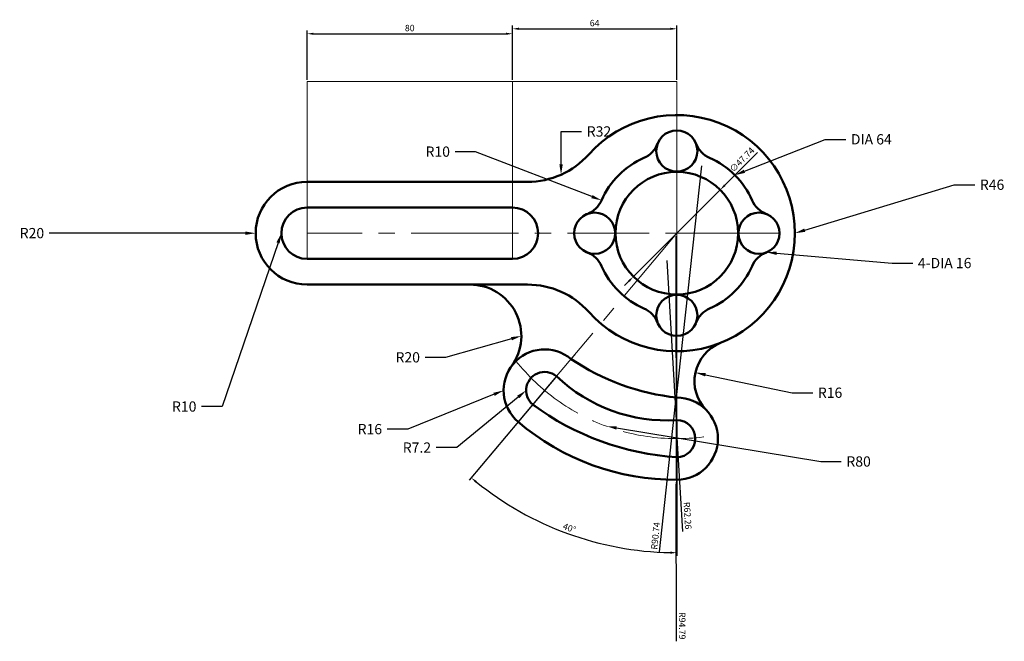
# Model space of a CAD drawing. Units: millimetres. Extents: x 2836 to 3220, y 1446 to 1688.
import ezdxf
from ezdxf import colors
from ezdxf.entities.mleader import LeaderData, LeaderLine
from ezdxf.math import Vec2, Vec3

# ---------------------------------------------------------------- set-up
doc = ezdxf.new("R2010")
doc.units = ezdxf.units.MM
doc.linetypes.add('CENTER', pattern=[50.8, 31.75, -6.35, 6.35, -6.35])
for name, color, linetype, lineweight in [('M-CNTR', 4, 'CENTER', 18), ('M-CONS', 8, 'Continuous', 13), ('M-DIMS', 2, 'Continuous', 25), ('M-OUTL', 7, 'Continuous', 50)]:
    doc.layers.add(name, color=color, linetype=linetype, lineweight=lineweight)
doc.styles.get("Standard").update_dxf_attribs({"font": 'arial.ttf'})
doc.dimstyles.new('ISO-25', dxfattribs={"dimtxt": 2.5, "dimasz": 2.5, "dimexe": 1.25, "dimexo": 0.625, "dimtad": 1, "dimtxsty": 'Standard', "dimcen": 2.5, "dimadec": 0, "dimazin": 0, "dimtfac": 1, "dimtmove": 0, "dimatfit": 3, "dimfxl": 1, "dimarcsym": 0})

# ---------------------------------------------------------------- blocks, each defined once
blk = doc.blocks.new('*U1')
blk.add_circle((0, 0), 8)
blk = doc.blocks.new('*U2')
at = {"layer": 'M-OUTL', "color": 0, "linetype": 'ByBlock', "lineweight": -2, "transparency": 16777216}
blk.add_blockref('*U1', (3092.05, 1637.01), dxfattribs=at)
for p, rotation in [((3060.05, 1605.01), 90), ((3124.05, 1605.01), 270), ((3092.05, 1573.01), 180)]:
    blk.add_blockref('*U1', p, dxfattribs=dict(at, rotation=rotation))
blk = doc.blocks.new('*D3')
at = {"layer": 'Defpoints', "color": 0, "transparency": 16777216}
for p in [(3028.05, 1682.68), (2948.05, 1664.13), (3028.05, 1664.13)]:
    blk.add_point(p, dxfattribs=at)
at = {"layer": 'M-DIMS', "color": 0, "lineweight": -2, "transparency": 16777216}
for p, q in [((2948.05, 1664.76), (2948.05, 1683.93)), ((3028.05, 1664.76), (3028.05, 1683.93)), ((2950.55, 1682.68), (3025.55, 1682.68))]:
    blk.add_line(p, q, dxfattribs=at)
at = {"layer": 'M-DIMS', "color": 0, "transparency": 16777216}
for points in [[(2950.55, 1683.09), (2950.55, 1682.26), (2948.05, 1682.68)], [(3025.55, 1683.09), (3025.55, 1682.26), (3028.05, 1682.68)]]:
    blk.add_solid(points, dxfattribs=at)
at = {"layer": 'M-DIMS', "color": 0, "transparency": 16777216, "insert": (2988.05, 1684.58), "char_height": 2.5, "attachment_point": 5}
blk.add_mtext('80', dxfattribs=at)
blk = doc.blocks.new('*D4')
at = {"layer": 'Defpoints', "color": 0, "transparency": 16777216}
for p in [(3092.05, 1684.61), (3028.05, 1664.13), (3092.05, 1664.13)]:
    blk.add_point(p, dxfattribs=at)
at = {"layer": 'M-DIMS', "color": 0, "lineweight": -2, "transparency": 16777216}
for p, q in [((3028.05, 1664.76), (3028.05, 1685.86)), ((3030.55, 1684.61), (3089.55, 1684.61)), ((3092.05, 1664.76), (3092.05, 1685.86))]:
    blk.add_line(p, q, dxfattribs=at)
at = {"layer": 'M-DIMS', "color": 0, "transparency": 16777216}
for points in [[(3030.55, 1685.03), (3030.55, 1684.19), (3028.05, 1684.61)], [(3089.55, 1685.03), (3089.55, 1684.19), (3092.05, 1684.61)]]:
    blk.add_solid(points, dxfattribs=at)
at = {"layer": 'M-DIMS', "color": 0, "transparency": 16777216, "insert": (3060.05, 1686.51), "char_height": 2.5, "attachment_point": 5}
blk.add_mtext('64', dxfattribs=at)
blk = doc.blocks.new('*D5')
at = {"layer": 'Defpoints', "color": 0, "transparency": 16777216}
for p in [(3092.05, 1605.01), (3092.05, 1559.01), (3045.21, 1549.28), (3092.05, 1532.21), (3036.15, 1493.86)]:
    blk.add_point(p, dxfattribs=at)
at = {"layer": 'M-DIMS', "color": 0, "lineweight": -2, "transparency": 16777216}
for p, q in [((3044.81, 1548.8), (3011.19, 1508.81)), ((3092.05, 1531.59), (3092.05, 1479.34))]:
    blk.add_line(p, q, dxfattribs=at)
blk.add_arc((3092.05, 1605.01), 124.42, 231.1062, 268.8487, dxfattribs=at)
at = {"layer": 'M-DIMS', "color": 0, "transparency": 16777216}
for points in [[(3013.66, 1507.85), (3014.19, 1508.5), (3012, 1509.76)], [(3089.55, 1481.04), (3089.54, 1480.2), (3092.05, 1480.59)]]:
    blk.add_solid(points, dxfattribs=at)
at = {"layer": 'M-DIMS', "color": 0, "transparency": 16777216, "insert": (3050.1, 1489.9), "char_height": 2.5, "attachment_point": 5, "rotation": 339.9775}
blk.add_mtext('40°', dxfattribs=at)
blk = doc.blocks.new('FLANGE-SCALLOP-R32')
for centre, radius, start, end in [((-3.61, 18.1), 10, 23.5565, 68.8316), ((34.89, 34.89), 32, 203.5565, 246.4435), ((18.1, -3.61), 10, 21.1684, 66.4435)]:
    blk.add_arc(centre, radius, start, end)
blk = doc.blocks.new('*D7')
at = {"layer": 'Defpoints', "color": 0, "transparency": 16777216}
for p in [(3108.93, 1621.89), (3075.17, 1588.14)]:
    blk.add_point(p, dxfattribs=at)
at = {"layer": 'M-DIMS', "color": 0, "lineweight": -2, "transparency": 16777216}
for p, q in [((3123.44, 1636.4), (3110.7, 1623.66)), ((3075.17, 1588.14), (3108.93, 1621.89)), ((3073.4, 1586.37), (3071.63, 1584.6))]:
    blk.add_line(p, q, dxfattribs=at)
at = {"layer": 'M-DIMS', "color": 0, "transparency": 16777216}
for points in [[(3110.4, 1623.95), (3110.99, 1623.36), (3108.93, 1621.89)], [(3073.11, 1586.66), (3073.7, 1586.07), (3075.17, 1588.14)]]:
    blk.add_solid(points, dxfattribs=at)
at = {"layer": 'M-DIMS', "color": 0, "transparency": 16777216, "insert": (3117.66, 1633.41), "char_height": 2.5, "attachment_point": 5, "rotation": 44.9932}
blk.add_mtext('∅47.74', dxfattribs=at)
blk = doc.blocks.new('*D8')
at = {"layer": 'Defpoints', "color": 0, "transparency": 16777216}
for p in [(3091.61, 1603.8), (3091.82, 1509.01)]:
    blk.add_point(p, dxfattribs=at)
at = {"layer": 'M-DIMS', "color": 0, "lineweight": -2, "transparency": 16777216}
for p, q in [((3091.61, 1603.8), (3091.82, 1509.01)), ((3091.96, 1446.1), (3091.83, 1506.51))]:
    blk.add_line(p, q, dxfattribs=at)
at = {"layer": 'M-DIMS', "color": 0, "transparency": 16777216}
blk.add_solid([(3092.24, 1506.51), (3091.41, 1506.51), (3091.82, 1509.01)], dxfattribs=at)
at = {"layer": 'M-DIMS', "color": 0, "transparency": 16777216, "insert": (3093.85, 1452.14), "char_height": 2.5, "attachment_point": 5, "rotation": 270.1296}
blk.add_mtext('R94.79', dxfattribs=at)
blk = doc.blocks.new('*D9')
at = {"layer": 'Defpoints', "color": 0, "transparency": 16777216}
for p in [(3101.61, 1631.25), (3091.82, 1541.04)]:
    blk.add_point(p, dxfattribs=at)
at = {"layer": 'M-DIMS', "color": 0, "lineweight": -2, "transparency": 16777216}
for p, q in [((3101.61, 1631.25), (3091.82, 1541.04)), ((3085.3, 1480.91), (3091.55, 1538.55))]:
    blk.add_line(p, q, dxfattribs=at)
at = {"layer": 'M-DIMS', "color": 0, "transparency": 16777216}
blk.add_solid([(3091.14, 1538.6), (3091.97, 1538.51), (3091.82, 1541.04)], dxfattribs=at)
at = {"layer": 'M-DIMS', "color": 0, "transparency": 16777216, "insert": (3084.06, 1487.12), "char_height": 2.5, "attachment_point": 5, "rotation": 83.8079}
blk.add_mtext('R90.74', dxfattribs=at)
blk = doc.blocks.new('*D10')
at = {"layer": 'Defpoints', "color": 0, "transparency": 16777216}
for p in [(3088.16, 1594.35), (3091.82, 1532.2)]:
    blk.add_point(p, dxfattribs=at)
at = {"layer": 'M-DIMS', "color": 0, "lineweight": -2, "transparency": 16777216}
for p, q in [((3088.16, 1594.35), (3091.82, 1532.2)), ((3094.37, 1488.88), (3091.97, 1529.7))]:
    blk.add_line(p, q, dxfattribs=at)
at = {"layer": 'M-DIMS', "color": 0, "transparency": 16777216}
blk.add_solid([(3092.38, 1529.73), (3091.55, 1529.68), (3091.82, 1532.2)], dxfattribs=at)
at = {"layer": 'M-DIMS', "color": 0, "transparency": 16777216, "insert": (3095.91, 1495.02), "char_height": 2.5, "attachment_point": 5, "rotation": 273.3663}
blk.add_mtext('R62.26', dxfattribs=at)

msp = doc.modelspace()

# ---------------------------------------------------------------- linework, layer by layer
at = {"layer": 'M-CNTR'}
for p, q in [((3092.049, 1605.013), (3092.049, 1664.134)), ((3092.049, 1664.134), (3092.049, 1549.257)), ((3092.049, 1549.257), (3092.049, 1606.695)), ((3020.316, 1605.013), (2948.049, 1605.013)), ((3132.049, 1605.013), (3020.316, 1605.013)), ((3092.049, 1605.013), (3045.21, 1549.281)), ((3092.049, 1605.013), (3132.049, 1605.013)), ((3052.59, 1558.063), (3050.872, 1556.018)), ((3092.049, 1559.013), (3092.049, 1532.213)), ((3045.21, 1549.281), (3030.283, 1531.521)), ((3092.049, 1532.213), (3092.049, 1509.013))]:
    msp.add_line(p, q, dxfattribs=at)
msp.add_arc((3092.049, 1605.013), 80, 218.47659, 281.47834, dxfattribs=at)
at = {"layer": 'M-CONS'}
for p, q in [((3028.049, 1664.134), (2948.049, 1664.134)), ((2948.049, 1664.134), (2948.049, 1595.013)), ((3092.049, 1664.134), (3028.049, 1664.134)), ((3028.049, 1664.134), (3028.049, 1595.013))]:
    msp.add_line(p, q, dxfattribs=at)
msp.add_arc((3092.049, 1605.013), 80, 194.47751, 194.66108, dxfattribs=at)
at = {"layer": 'M-OUTL'}
for p, q in [((2948.049, 1625.013), (3033.911, 1625.013)), ((2948.049, 1615.013), (3028.049, 1615.013)), ((2948.049, 1595.013), (3028.049, 1595.013)), ((2948.049, 1585.013), (3033.911, 1585.013))]:
    msp.add_line(p, q, dxfattribs=at)
msp.add_circle((3092.049, 1605.013), 23.868, dxfattribs=at)
for centre, radius, start, end in [((3092.049, 1605.013), 46, 221.81031, 138.18969), ((3033.911, 1657.013), 32, 270, 318.18969), ((2948.049, 1605.013), 20, 90, 270), ((2948.049, 1605.013), 10, 90, 270), ((3028.049, 1605.013), 10, 270, 90), ((3011.513, 1565.013), 20, 323.83691, 90), ((3033.911, 1553.013), 32, 41.81031, 90), ((3114.926, 1547.388), 16, 111.65301, 224.36436), ((3040.577, 1543.769), 16, 49.95493, 229.95493), ((3101.609, 1631.247), 90.739, 236.00275, 263.95218), ((3040.577, 1543.769), 7.2, 49.95493, 237.73801), ((3088.164, 1594.354), 62.262, 226.37816, 273.57677), ((3098.739, 1623.373), 105.773, 233.58177, 266.37316), ((3092.049, 1525.013), 16, 270, 90), ((3091.606, 1603.797), 94.786, 229.68718, 270.26775), ((3092.049, 1525.013), 7.2, 270, 90)]:
    msp.add_arc(centre, radius, start, end, dxfattribs=at)

# ---------------------------------------------------------------- block references
for name, p in [('*U2', (0, 0)), ('FLANGE-SCALLOP-R32', (3057.16, 1570.124))]:
    msp.add_blockref(name, p, dxfattribs=at)
for p, rotation in [((3057.16, 1639.901), 270.0000000000019), ((3126.937, 1639.901), 180), ((3126.937, 1570.124), 90.00000000000095)]:
    msp.add_blockref('FLANGE-SCALLOP-R32', p, dxfattribs=dict(at, rotation=rotation))

# ---------------------------------------------------------------- dimensions: what is measured, and where the dimension line sits
at = {"layer": 'M-DIMS'}
for base, p1, p2, picture, middle in [((3092.049, 1684.609), (3028.049, 1664.134), (3092.049, 1664.134), '*D4', (3060.049, 1686.51)), ((3028.049, 1682.677), (2948.049, 1664.134), (3028.049, 1664.134), '*D3', (2988.049, 1684.578))]:
    dim = msp.add_linear_dim(base=base, p1=p1, p2=p2, dimstyle='ISO-25', override={"dimclrd": 0, "dimclre": 0, "dimclrt": 0}, dxfattribs=at)
    dim.commit()
    dim.dimension.update_dxf_attribs({"geometry": picture, "text_midpoint": middle})
dim = msp.add_diameter_dim_2p(p1=(3075.169, 1588.137), p2=(3108.928, 1621.888), dimstyle='ISO-25', override={"dimdec": 2, "dimlfac": 1, "dimrnd": 0, "dimzin": 0, "dimdsep": 46, "dimlunit": 2}, dxfattribs=at)
dim.commit()
dim.dimension.update_dxf_attribs({"geometry": '*D7', "text_midpoint": (3119.056, 1632.013), "dimtype": 163})
for center, mpoint, picture, middle in [((3101.609, 1631.247), (3091.821, 1541.037), '*D9', (3085.949, 1486.911)), ((3091.606, 1603.797), (3091.82, 1509.012), '*D8', (3091.949, 1452.141)), ((3088.164, 1594.354), (3091.82, 1532.199), '*D10', (3094.014, 1494.906))]:
    dim = msp.add_radius_dim(center=center, mpoint=mpoint, dimstyle='ISO-25', override={"dimdec": 2, "dimlfac": 1, "dimrnd": 0, "dimzin": 0, "dimdsep": 46, "dimlunit": 2}, dxfattribs=at)
    dim.commit()
    dim.dimension.update_dxf_attribs({"geometry": picture, "text_midpoint": middle, "dimtype": 164})
dim = msp.add_angular_dim_2l(base=(3036.151, 1493.857), line1=((3092.049, 1559.013), (3092.049, 1532.213)), line2=((3092.049, 1605.013), (3045.21, 1549.281)), dimstyle='ISO-25', override={"dimclrd": 0, "dimclre": 0, "dimclrt": 0}, dxfattribs=at)
dim.commit()
dim.dimension.update_dxf_attribs({"geometry": '*D5', "text_midpoint": (3050.1, 1489.9)})

# ---------------------------------------------------------------- leaders
ml = msp.add_multileader_mtext('Standard', dxfattribs=at)
ml.set_content('R32', color=256)
ml.set_leader_properties()
ml.build(insert=Vec2(0, 0))
ctx = ml.context
ctx.base_point, ctx.plane_origin = Vec3(3054.975, 1644.6), Vec3(3046.975, 1627.801)
notes = []
notes.append((ctx, [(0, (1, 1, 0), (3046.975, 1644.6), (1, 0), 8, [(0, [(3046.975, 1627.801)], 0, [])])]))
ctx.mtext.insert, ctx.mtext.flow_direction = Vec3(3056.975, 1646.636), 5
ml = msp.add_multileader_mtext('Standard', dxfattribs=at)
ml.set_content('DIA 64', color=256)
ml.set_leader_properties()
ml.build(insert=Vec2(0, 0))
ctx = ml.context
ctx.base_point, ctx.plane_origin = Vec3(3157.82, 1641.544), Vec3(3114.676, 1627.64)
notes.append((ctx, [(0, (1, 1, 0), (3149.82, 1641.544), (1, 0), 8, [(0, [(3114.676, 1627.64)], 0, [])])]))
ctx.mtext.insert, ctx.mtext.flow_direction = Vec3(3159.82, 1643.578), 5
ml = msp.add_multileader_mtext('Standard', dxfattribs=at)
ml.set_content('R10', color=256)
ml.set_leader_properties()
ml.build(insert=Vec2(0, 0))
ctx = ml.context
ctx.base_point, ctx.plane_origin = Vec3(2992.169, 1636.742), Vec3(3062.715, 1617.801)
ctx.text_align_type = 2
notes.append((ctx, [(0, (1, 1, 0), (3013.714, 1636.742), (-1, 0), 8, [(0, [(3062.715, 1617.801)], 0, [])])]))
ctx.mtext.insert, ctx.mtext.alignment, ctx.mtext.flow_direction = Vec3(3003.714, 1638.776), 3, 5
ml = msp.add_multileader_mtext('Standard', dxfattribs=at)
ml.set_content('R46', color=256)
ml.set_leader_properties()
ml.build(insert=Vec2(0, 0))
ctx = ml.context
ctx.base_point, ctx.plane_origin = Vec3(3208.067, 1623.862), Vec3(3138.049, 1605.013)
notes.append((ctx, [(0, (1, 1, 0), (3200.067, 1623.862), (1, 0), 8, [(0, [(3138.049, 1605.013)], 0, [])])]))
ctx.mtext.insert, ctx.mtext.flow_direction = Vec3(3210.067, 1625.896), 5
ml = msp.add_multileader_mtext('Standard', dxfattribs=at)
ml.set_content('R20', color=256)
ml.set_leader_properties()
ml.build(insert=Vec2(0, 0))
ctx = ml.context
ctx.base_point, ctx.plane_origin = Vec3(2834.124, 1605.013), Vec3(2928.049, 1605.013)
ctx.text_align_type = 2
notes.append((ctx, [(0, (1, 1, 0), (2855.669, 1605.013), (-1, 0), 8, [(0, [(2928.049, 1605.013)], 0, [])])]))
ctx.mtext.insert, ctx.mtext.alignment, ctx.mtext.flow_direction = Vec3(2845.669, 1607.047), 3, 5
ml = msp.add_multileader_mtext('Standard', dxfattribs=at)
ml.set_content('R10', color=256)
ml.set_leader_properties()
ml.build(insert=Vec2(0, 0))
ctx = ml.context
ctx.base_point, ctx.plane_origin = Vec3(2893.436, 1537.485), Vec3(2938.049, 1605.013)
ctx.text_align_type = 2
notes.append((ctx, [(0, (1, 1, 0), (2914.981, 1537.485), (-1, 0), 8, [(0, [(2938.049, 1605.013)], 0, [])])]))
ctx.mtext.insert, ctx.mtext.alignment, ctx.mtext.flow_direction = Vec3(2904.981, 1539.519), 3, 5
ml = msp.add_multileader_mtext('Standard', dxfattribs=at)
ml.set_content('4-DIA 16', color=256)
ml.set_leader_properties()
ml.build(insert=Vec2(0, 0))
ctx = ml.context
ctx.base_point, ctx.plane_origin = Vec3(3183.923, 1593.362), Vec3(3126.937, 1597.552)
notes.append((ctx, [(0, (1, 1, 0), (3175.923, 1593.362), (1, 0), 8, [(0, [(3126.937, 1597.552)], 0, [])])]))
ctx.mtext.insert, ctx.mtext.flow_direction = Vec3(3185.923, 1595.396), 5
ml = msp.add_multileader_mtext('Standard', dxfattribs=at)
ml.set_content('R20', color=256)
ml.set_leader_properties()
ml.build(insert=Vec2(0, 0))
ctx = ml.context
ctx.base_point, ctx.plane_origin = Vec3(2980.483, 1556.653), Vec3(3031.513, 1565.013)
ctx.text_align_type = 2
notes.append((ctx, [(0, (1, 1, 0), (3002.027, 1556.653), (-1, 0), 8, [(0, [(3031.513, 1565.013)], 0, [])])]))
ctx.mtext.insert, ctx.mtext.alignment, ctx.mtext.flow_direction = Vec3(2992.027, 1558.687), 3, 5
ml = msp.add_multileader_mtext('Standard', dxfattribs=at)
ml.set_content('R16', color=256)
ml.set_leader_properties()
ml.build(insert=Vec2(0, 0))
ctx = ml.context
ctx.base_point, ctx.plane_origin = Vec3(3144.972, 1542.869), Vec3(3099.275, 1550.712)
notes.append((ctx, [(0, (1, 1, 0), (3136.972, 1542.869), (1, 0), 8, [(0, [(3099.275, 1550.712)], 0, [])])]))
ctx.mtext.insert, ctx.mtext.flow_direction = Vec3(3146.972, 1544.903), 5
ml = msp.add_multileader_mtext('Standard', dxfattribs=at)
ml.set_content('R16', color=256)
ml.set_leader_properties()
ml.build(insert=Vec2(0, 0))
ctx = ml.context
ctx.base_point, ctx.plane_origin = Vec3(2965.72, 1528.69), Vec3(3024.577, 1543.769)
ctx.text_align_type = 2
notes.append((ctx, [(0, (1, 1, 0), (2987.275, 1528.69), (-1, 0), 8, [(0, [(3024.577, 1543.769)], 0, [])])]))
ctx.mtext.insert, ctx.mtext.alignment, ctx.mtext.flow_direction = Vec3(2977.275, 1530.724), 3, 5
ml = msp.add_multileader_mtext('Standard', dxfattribs=at)
ml.set_content('R7.2', color=256)
ml.set_leader_properties()
ml.build(insert=Vec2(0, 0))
ctx = ml.context
ctx.base_point, ctx.plane_origin = Vec3(2983.297, 1521.536), Vec3(3033.377, 1543.769)
ctx.text_align_type = 2
notes.append((ctx, [(0, (1, 1, 0), (3006.366, 1521.536), (-1, 0), 8, [(0, [(3033.377, 1543.769)], 0, [])])]))
ctx.mtext.insert, ctx.mtext.alignment, ctx.mtext.flow_direction = Vec3(2996.366, 1523.536), 3, 5
ml = msp.add_multileader_mtext('Standard', dxfattribs=at)
ml.set_content('R80', color=256)
ml.set_leader_properties()
ml.build(insert=Vec2(0, 0))
ctx = ml.context
ctx.base_point, ctx.plane_origin = Vec3(3156.085, 1516.089), Vec3(3064.657, 1529.848)
notes.append((ctx, [(0, (1, 1, 0), (3148.085, 1516.089), (1, 0), 8, [(0, [(3064.657, 1529.848)], 0, [])])]))
ctx.mtext.insert, ctx.mtext.flow_direction = Vec3(3158.085, 1518.123), 5
for ctx, leaders in notes:
    for number, flags, end, landing, length, lines in leaders:
        leader = LeaderData()
        leader.index, (leader.has_last_leader_line, leader.has_dogleg_vector, leader.attachment_direction) = number, flags
        leader.last_leader_point, leader.dogleg_vector, leader.dogleg_length = Vec3(end), Vec3(landing), length
        for number, points, colour, breaks in lines:
            line = LeaderLine()
            line.index, line.vertices, line.color, line.breaks = number, Vec3.list(points), colors.encode_raw_color(colour), breaks
            leader.lines.append(line)
        ctx.leaders.append(leader)

doc.saveas('drawing.dxf')
